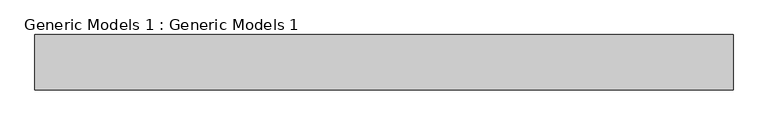
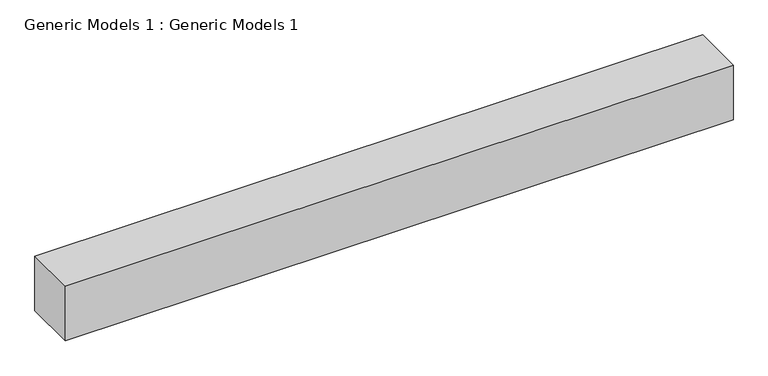
"""IFC4 building model written with IfcOpenShell, lengths in millimetres: proxy geometry, Generic Models 1 : Generic Models 1."""

from ifc_helpers import new_model, si_unit, frame, origin, place, context, project, spatial, polyline, outline, extrude, source, transform, mapped, element, save


def generic_models_1_generic_models_1_a4a6df41(model_context):
    return source(origin(), model_context, "Body", "SweptSolid", [
        extrude(outline(polyline([(4163.3104739, -8641.1821053), (4163.3104739, -9760.0213812), (-9959.1625896, -9760.0213812), (-9959.1625896, -8641.1821053), (4163.3104739, -8641.1821053)])), frame((0.0, 0.0, 2562.8995622), z_axis=(0.0, 0.0, 1.0), x_axis=(1.0, 0.0, 0.0)), (0.0, 0.0, 1.0), 1222.0313984),
    ])


if __name__ == "__main__":
    model = new_model("IFC4")
    model_context = context("Model", 3, world=origin())
    ifc_project = project(units=[si_unit("LENGTHUNIT", "METRE", prefix="MILLI")], contexts=[model_context])
    site = spatial("IfcSite", under=ifc_project)
    building = spatial("IfcBuilding", under=site)
    placement = place(None, origin())
    generic_models_1_generic_models_1_shape = generic_models_1_generic_models_1_a4a6df41(model_context)
    element("IfcBuildingElementProxy", 1, Name="Generic Models 1 : Generic Models 1", ObjectType="Generic Models 1 : Generic Models 1", at=placement, inside=building, context=model_context, shape_type="MappedRepresentation", body=[
        mapped(generic_models_1_generic_models_1_shape, transform((0.0, 0.0, 0.0), x_axis=(1.0, 0.0, 0.0), y_axis=(0.0, 1.0, 0.0), z_axis=(0.0, 0.0, 1.0))),
    ])
    save(model, "model.ifc")
